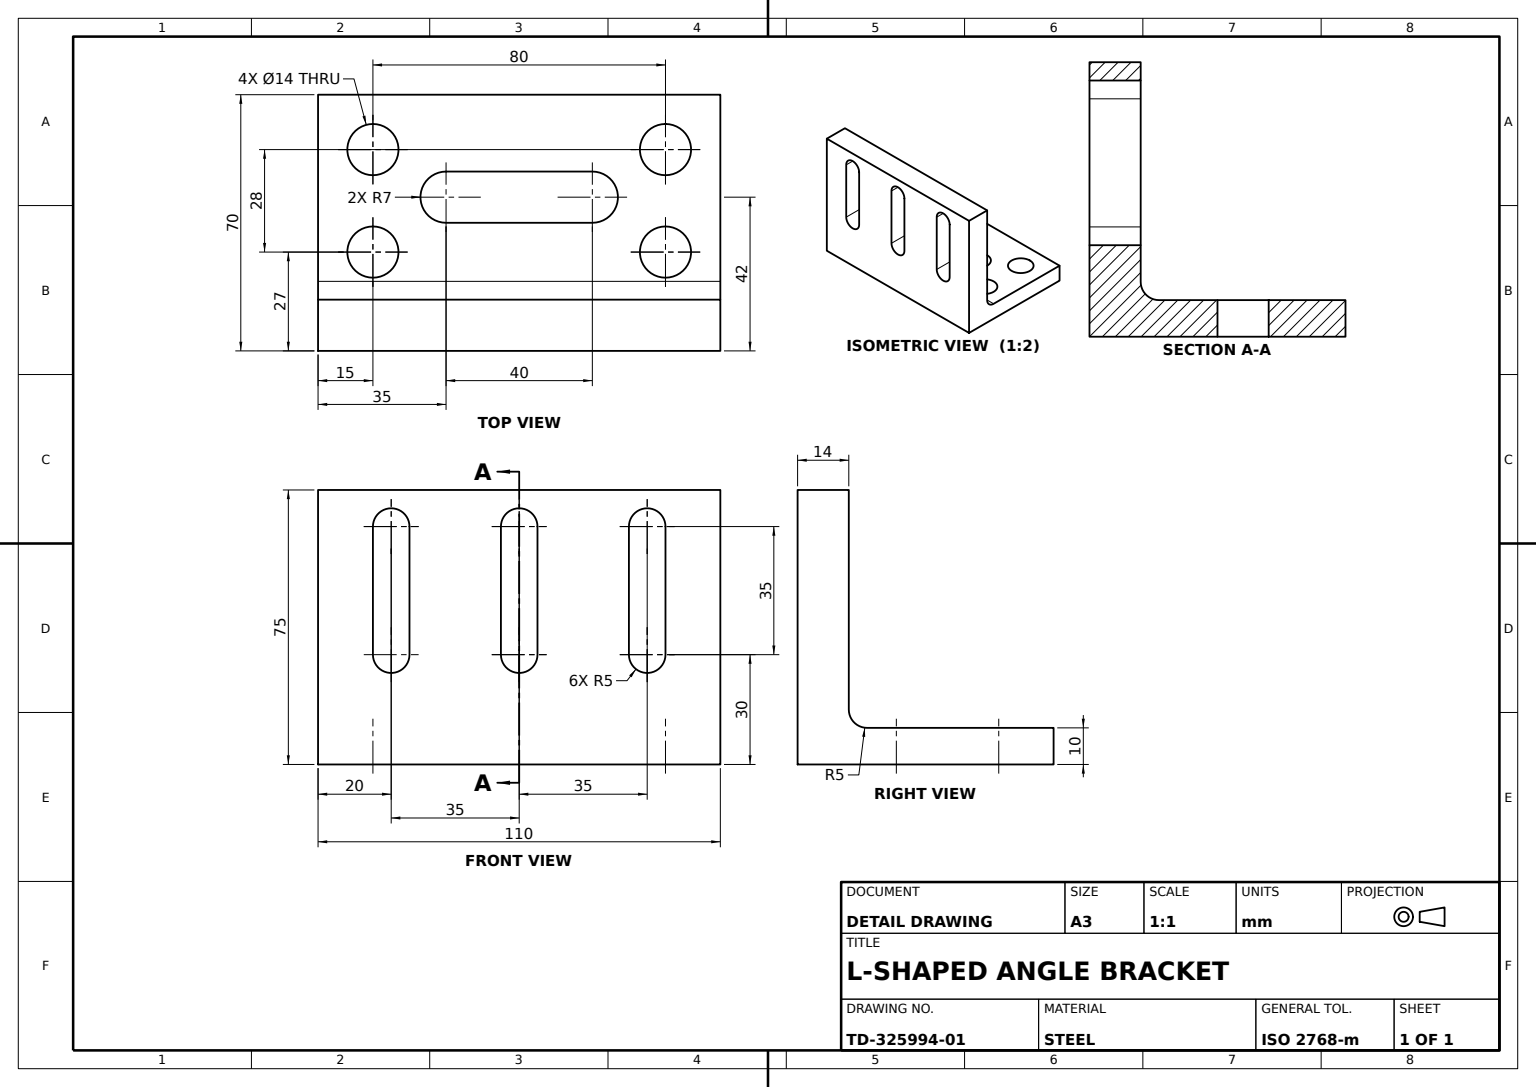
SolidWorks part; units mm, degrees
material "Plain Carbon Steel"
ref_plane "Front Plane" through (0, 0, 0) normal (0, 0, 1) x (1, 0, 0)
ref_plane "Top Plane" through (0, 0, 0) normal (0, 1, 0) x (1, 0, 0)
ref_plane "Right Plane" through (0, 0, 0) normal (1, 0, 0) x (0, 0, -1)
sketch "Bracket L-Profile Sketch" plane through (0, 0, 0) normal (1, 0, 0) x (0, 0, -1)
  line L0 (0, 0) -> (0, 75)
  line L1 (0, 75) -> (14, 75)
  line L2 (14, 75) -> (14, 10)
  line L3 (14, 10) -> (70, 10)
  line L4 (70, 10) -> (70, 0)
  line L5 (70, 0) -> (0, 0)
  dimension "D1" = 70
  dimension "D2" = 75
  dimension "D3" = 14
  dimension "D4" = 10
extrude "L-Bracket Body" add sketch "Bracket L-Profile Sketch" against normal blind 110
sketch "Vertical Leg Slots Sketch" plane through (0, 0, -14) normal (0, 0, -1) x (-1, 0, 0)
  line L0 (15, 65) -> (15, 30)
  line L1 (25, 30) -> (25, 65)
  line L2 (50, 65) -> (50, 30)
  line L3 (60, 30) -> (60, 65)
  line L4 (85, 65) -> (85, 30)
  line L5 (95, 30) -> (95, 65)
  line L6 (110, 75) -> (0, 75) construction
  arc A0 (15, 30) -> (25, 30) centre (20, 30) ccw
  arc A1 (25, 65) -> (15, 65) centre (20, 65) ccw
  arc A2 (50, 30) -> (60, 30) centre (55, 30) ccw
  arc A3 (60, 65) -> (50, 65) centre (55, 65) ccw
  arc A4 (85, 30) -> (95, 30) centre (90, 30) ccw
  arc A5 (95, 65) -> (85, 65) centre (90, 65) ccw
  dimension "D4" = 5
  dimension "D5" = 5
  dimension "D6" = 5
  dimension "D1" = 20
  dimension "D2" = 20
  dimension "D3" = 35
  dimension "D7" = 10
  dimension "D8" = 10
  dimension "D9" = 10
  dimension "D10" = 35
  dimension "D11" = 35
  dimension "D12" = 35
extrude "Vertical Leg Slots 3x10" cut sketch "Vertical Leg Slots Sketch" against normal blind 110
sketch "Base Holes Sketch" plane through (0, 10, 0) normal (0, 1, 0) x (1, 0, 0)
  line L0 (-110, 70) -> (-110, 14) construction
  line L1 (0, 70) -> (0, 14) construction
  line L2 (-110, 42) -> (0, 42) construction
  line L3 (-75, 49) -> (-35, 49)
  line L4 (-35, 35) -> (-75, 35)
  circle A0 centre (-95, 55) radius 7
  circle A1 centre (-15, 55) radius 7
  circle A2 centre (-15, 27) radius 7
  circle A3 centre (-95, 27) radius 7
  arc A4 (-35, 49) -> (-35, 35) centre (-35, 42) cw
  arc A5 (-75, 35) -> (-75, 49) centre (-75, 42) cw
  dimension "D1" = 14
  dimension "D2" = 15
  dimension "D7" = 7
  dimension "D3" = 28
  dimension "D4" = 15
  dimension "D5" = 15
  dimension "D6" = 40
  dimension "D8" = 35
extrude "Base Mounting Holes" cut sketch "Base Holes Sketch" against normal blind 110
fillet "Inner Corner Fillet R5" radius 5 1 edges at (-55, 10, -14)
